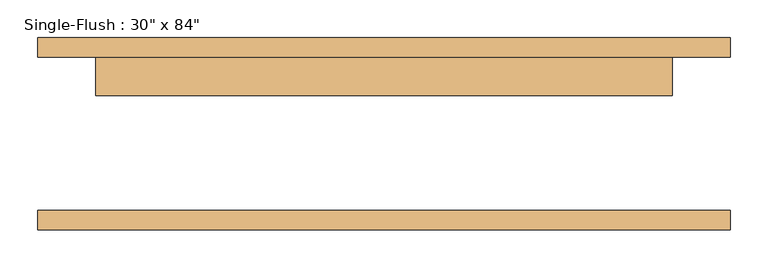
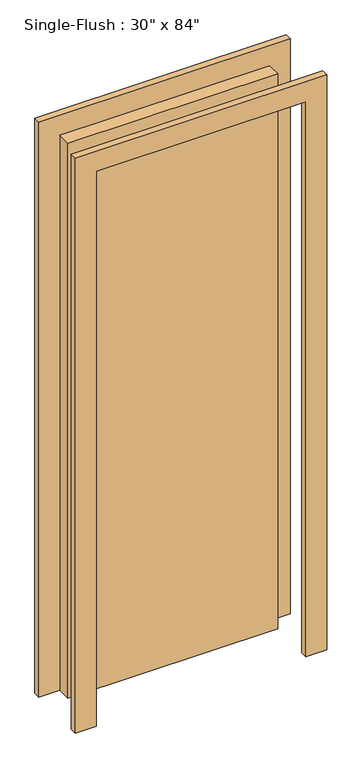
"""IFC4 building model written with IfcOpenShell, lengths in millimetres: door geometry."""

from ifc_helpers import new_model, si_unit, frame, origin, origin_with_axes, place, context, project, spatial, polyline, outline, extrude, source, transform, mapped, element, save


def door_b6acaa4e(model_context):
    return source(origin(), model_context, "Body", "SweptSolid", [
        extrude(outline(polyline([(2209.8, -457.2), (0.0, -457.2), (0.0, -381.0), (2133.6, -381.0), (2133.6, 381.0), (0.0, 381.0), (0.0, 457.2), (2209.8, 457.2), (2209.8, -457.2)])), frame((0.0, 101.6, 0.0), z_axis=(0.0, 1.0, 0.0), x_axis=(0.0, 0.0, 1.0)), (0.0, 0.0, 1.0), 25.4),
        extrude(outline(polyline([(2209.8, 457.2), (2209.8, -457.2), (0.0, -457.2), (0.0, -381.0), (2133.6, -381.0), (2133.6, 381.0), (0.0, 381.0), (0.0, 457.2), (2209.8, 457.2)])), frame((0.0, -127.0, 0.0), z_axis=(0.0, 1.0, 0.0), x_axis=(0.0, 0.0, 1.0)), (0.0, 0.0, 1.0), 25.4),
        extrude(outline(polyline([(381.0, 50.8), (-381.0, 50.8), (-381.0, 101.6), (381.0, 101.6), (381.0, 50.8)])), origin_with_axes(), (0.0, 0.0, 1.0), 2133.6),
    ])


if __name__ == "__main__":
    model = new_model("IFC4")
    model_context = context("Model", 3, world=origin())
    ifc_project = project(units=[si_unit("LENGTHUNIT", "METRE", prefix="MILLI")], contexts=[model_context])
    site = spatial("IfcSite", under=ifc_project)
    building = spatial("IfcBuilding", under=site)
    placement = place(None, origin())
    door_shape = door_b6acaa4e(model_context)
    element("IfcDoor", 1, ObjectType="Single-Flush : 30\" x 84\"", at=placement, inside=building, context=model_context, shape_type="MappedRepresentation", body=[
        mapped(door_shape, transform((0.0, 0.0, 0.0), x_axis=(1.0, 0.0, 0.0), y_axis=(0.0, 1.0, 0.0), z_axis=(0.0, 0.0, 1.0))),
    ])
    save(model, "model.ifc")

# Revit data of these elements
# Type "Single-Flush : 30\" x 84\""
#   Type Mark = "4"
#   Construction Type Id = "MDOOR"
#   Assembly Code = "C1020"
#   Analytic Construction = "Metal"
#   Thickness = 0' - 2"
#   Heat Transfer Coefficient (U) = 0.651978 BTU/(h·ft²·°F)
#   Height = 7' - 0"
#   Trim Projection Ext = 0' - 1"
#   Trim Projection Int = 0' - 1"
#   Trim Width = 0' - 3"
#   Width = 2' - 6"
#   Define Thermal Properties by = 1
#   Door Material = Door - Panel
#   Frame Material = Door - Frame
#   Visual Light Transmittance = 0
#   Solar Heat Gain Coefficient = 0
#   Function = (empty or 0)
#   Wall Closure = (empty or 0)
# Element 1 (IfcDoor, "Single-Flush : 30\" x 84\"")
#   Materials on its faces: "Door - Frame", "Door - Panel"
# Materials
#   "Door - Panel": class "Wood", colour RGB 210 159 95, transparency 0
#   "Door - Frame": colour RGB 118 70 51, transparency 0
